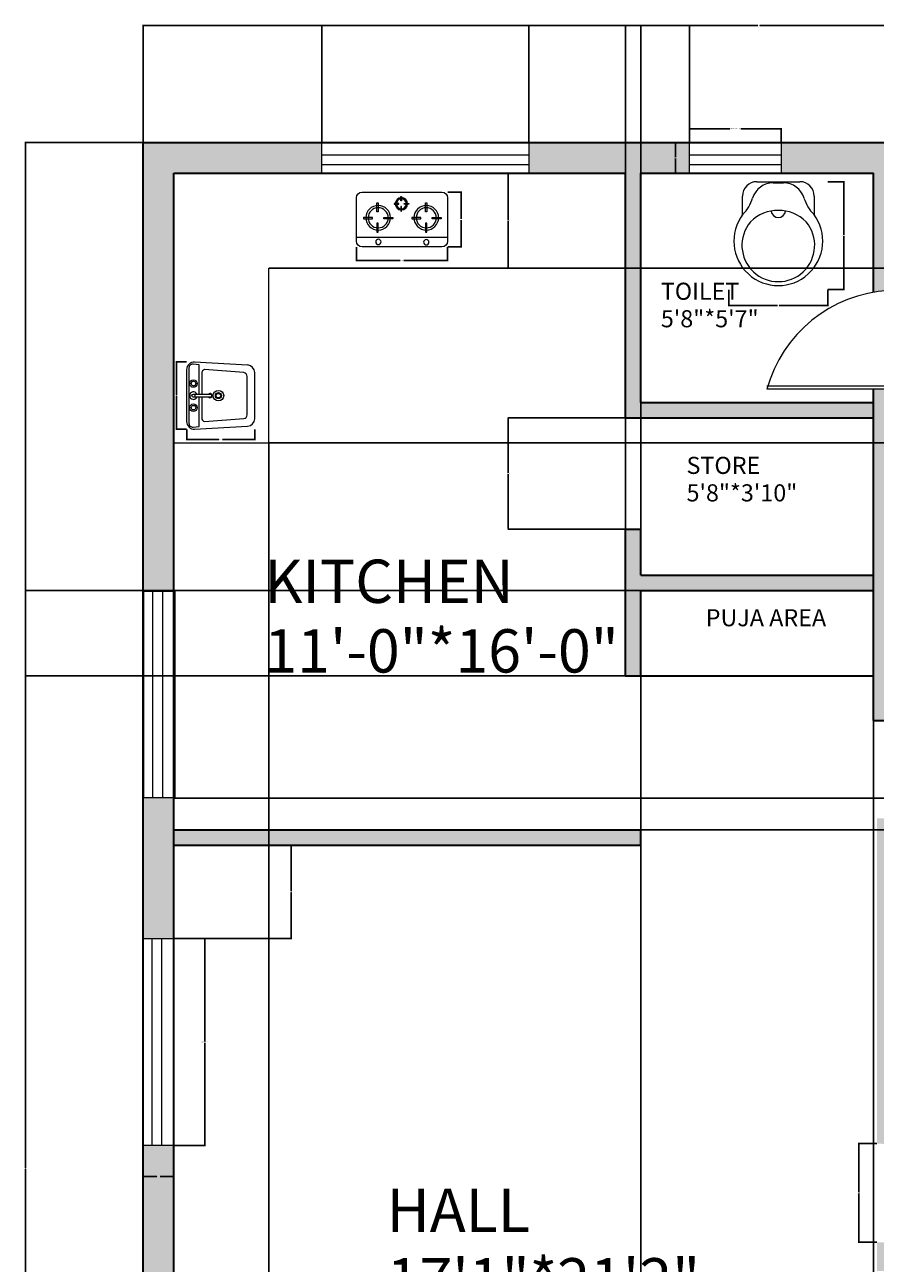
# Model space of a CAD drawing. Units: feet. Extents: x 2516 to 2945, y 1283 to 1993.
# Tile 2 of 3: x 2516 to 2764, y 1631 to 1993. Entities that reach past the tile are written whole.
import ezdxf

# ---------------------------------------------------------------- set-up
doc = ezdxf.new("R2010")
doc.units = ezdxf.units.FT
doc.layers.get('0').update_dxf_attribs({"lineweight": 18})
for name, color, linetype, lineweight in [('A-ANNO-DIMS', 2, 'Continuous', 18), ('A-AREA-IDEN', 7, 'Continuous', 18), ('A-EQPM', 8, 'Continuous', 18), ('A-FLOR-CASE', 8, 'Continuous', 18), ('A-FLOR-FIXT', 8, 'Continuous', 18), ('A-WALL', 7, 'Continuous', 35), ('A-WALL-PATT', 143, 'Continuous', 13), ('doors', 163, 'Continuous', 18), ('windows', 10, 'Continuous', 18)]:
    doc.layers.add(name, color=color, linetype=linetype, lineweight=lineweight)
doc.styles.get("Standard").update_dxf_attribs({"font": 'arial.ttf'})
doc.dimstyles.get("Standard").update_dxf_attribs({"dimtxt": 0.18, "dimasz": 0.18, "dimexe": 0.18, "dimexo": 0.0625, "dimgap": 0.09, "dimtad": 0, "dimtih": 1, "dimtoh": 1, "dimdec": 4, "dimzin": 0, "dimdsep": 46, "dimtxsty": 'Standard', "dimcen": 0.09, "dimadec": 0, "dimazin": 0, "dimtfac": 1, "dimtdec": 4, "dimtofl": 0, "dimtmove": 0, "dimatfit": 3, "dimfxl": 1, "dimtolj": 1, "dimtzin": 0, "dimarcsym": 0})

# ---------------------------------------------------------------- blocks, each defined once
blk = doc.blocks.new('door')
at = {"layer": 'doors'}
for p, q in [((-0.98, 0), (-0.98, 35.67)), ((0, 35.67), (0, 0)), ((-0.98, 0), (27.91, 0))]:
    blk.add_line(p, q, dxfattribs=at)
blk.add_arc((-11.23, -2.17), 39.2, 3.167, 74.8469, dxfattribs=at)
blk = doc.blocks.new('A$C39AA428E')
for p, q in [((0.4054, 0.435), (0.0392, 0.435)), ((0.3942, 0.45), (0.0499, 0.45)), ((0, 0.3972), (0.0194, 0.0472)), ((0.0143, 0.408), (0.0177, 0.3665)), ((0.0177, 0.3665), (0.2121, 0.3665)), ((0.05, 0.3311), (0.0702, 0.0729)), ((0.2121, 0.35), (0.0742, 0.35)), ((0.2121, 0.285), (0.2121, 0.405)), ((0.2321, 0.405), (0.2321, 0.285)), ((0.2321, 0.3665), (0.4265, 0.3665)), ((0.3699, 0.35), (0.2321, 0.35)), ((0.374, 0.0729), (0.3941, 0.3311)), ((0.4247, 0.0472), (0.4441, 0.3972)), ((0.4265, 0.3665), (0.4303, 0.4077)), ((0.2321, 0.285), (0.2121, 0.285)), ((0.0694, 0), (0.3748, 0)), ((0.0951, 0.05), (0.3491, 0.05))]:
    blk.add_line(p, q)
for centre, radius in [((0.1421, 0.405), 0.025), ((0.1421, 0.405), 0.015), ((0.2221, 0.405), 0.01), ((0.3021, 0.405), 0.025), ((0.3021, 0.405), 0.015), ((0.2221, 0.24), 0.035), ((0.2221, 0.24), 0.02), ((0.2221, 0.24), 0.015)]:
    blk.add_circle(centre, radius)
for centre, radius, start, end in [((0.0499, 0.4), 0.05, 90, 183.17983), ((0.0392, 0.41), 0.025, 90, 184.67219), ((0.2221, 0.405), 0.025, 293.57818, 246.42182), ((0.3942, 0.4), 0.05, 356.82017, 90), ((0.4054, 0.41), 0.025, 354.70992, 90), ((0.0742, 0.325), 0.025, 90, 165.81434), ((0.3699, 0.325), 0.025, 14.18566, 90), ((0.2221, 0.295), 0.0142, 134.62622, 45.19255), ((0.0694, 0.05), 0.05, 183.17983, 270), ((0.0951, 0.075), 0.025, 184.76364, 270), ((0.3491, 0.075), 0.025, 270, 355.23636), ((0.3748, 0.05), 0.05, 270, 356.82017)]:
    blk.add_arc(centre, radius, start, end)
blk = doc.blocks.new('A$C6EF51710')
at = {"linetype": 'ByBlock'}
for p, q in [((0.0508, 0.2843), (0.1169, 0.2843)), ((0, 0.0811), (0, 0.2335)), ((0.0041, 0.1392), (0.0041, 0.1755)), ((0.1169, 0.0303), (0.0508, 0.0303))]:
    blk.add_line(p, q, dxfattribs=at)
for centre, radius, start, end in [((0.2107, 0.1573), 0.1576, 232.8984, 127.1016), ((0.0508, 0.2335), 0.0508, 90, 180), ((0.0168, 0.3818), 0.1397, 287.1046, 315), ((0.2254, 0.1573), 0.1289, 230.0084, 129.9916), ((0.0803, 0.1755), 0.0762, 107.1046, 180), ((0.2413, 0.1573), 0.1397, 135, 225), ((0.1016, 0.1573), 0.0254, 275.2159, 84.7841), ((0.0803, 0.1392), 0.0762, 180, 252.8954), ((0.0508, 0.0811), 0.0508, 180, 270), ((0.0168, -0.0672), 0.1397, 45, 72.8954)]:
    blk.add_arc(centre, radius, start, end, dxfattribs=at)
blk = doc.blocks.new('A$C03A44EBA')
at = {"rotation": 270}
blk.add_blockref('A$C6EF51710', (0.0003, 0.3683), dxfattribs=at)
blk = doc.blocks.new('A$C2A3C6842')
for p, q in [((45, 432), (675, 432)), ((351.6, 363.3), (351.6, 398.9)), ((351.6, 398.9), (357.3, 398.9)), ((357.3, 398.9), (357.3, 363.3)), ((0, 45), (0, 387)), ((161.8, 346.9), (173.2, 346.9)), ((161.8, 275.6), (161.8, 346.9)), ((173.2, 346.9), (173.2, 275.6)), ((298.4, 341.9), (298.4, 336.2)), ((334, 341.9), (298.4, 341.9)), ((298.4, 336.2), (334, 336.2)), ((334, 336.2), (334, 341.9)), ((357.3, 363.3), (351.6, 363.3)), ((357.3, 318.8), (351.6, 318.8)), ((351.6, 318.8), (351.6, 283.1)), ((357.3, 283.1), (357.3, 318.8)), ((378.5, 336.2), (378.5, 341.9)), ((378.5, 341.9), (414.2, 341.9)), ((414.2, 336.2), (378.5, 336.2)), ((414.2, 341.9), (414.2, 336.2)), ((544.7, 346.9), (556.1, 346.9)), ((544.7, 275.6), (544.7, 346.9)), ((556.1, 346.9), (556.1, 275.6)), ((720, 387), (720, 45)), ((55.3, 232.9), (55.3, 221.5)), ((126.6, 232.9), (55.3, 232.9)), ((55.3, 221.5), (126.6, 221.5)), ((126.6, 221.5), (126.6, 232.9)), ((173.2, 275.6), (161.8, 275.6)), ((215.6, 221.5), (215.6, 232.9)), ((215.6, 232.9), (286.9, 232.9)), ((286.9, 221.5), (215.6, 221.5)), ((286.9, 232.9), (286.9, 221.5)), ((351.6, 283.1), (357.3, 283.1)), ((438.2, 232.9), (438.2, 221.5)), ((509.5, 232.9), (438.2, 232.9)), ((438.2, 221.5), (509.5, 221.5)), ((509.5, 221.5), (509.5, 232.9)), ((556.1, 275.6), (544.7, 275.6)), ((598.5, 232.9), (669.8, 232.9)), ((598.5, 221.5), (598.5, 232.9)), ((669.8, 221.5), (598.5, 221.5)), ((669.8, 232.9), (669.8, 221.5)), ((173.2, 186.6), (161.8, 186.6)), ((161.8, 186.6), (161.8, 115.3)), ((161.8, 115.3), (173.2, 115.3)), ((173.2, 115.3), (173.2, 186.6)), ((556.1, 186.6), (544.7, 186.6)), ((544.7, 186.6), (544.7, 115.3)), ((544.7, 115.3), (556.1, 115.3)), ((556.1, 115.3), (556.1, 186.6)), ((1.2, 76.7), (719.9, 76.7)), ((675, 0), (45, 0))]:
    blk.add_line(p, q)
at = {"extrusion": (0, -1e-16, -1)}
for centre, major_axis, start_param, end_param in [((45, 387), (31.8, 31.8), 3.926991, 5.497787), ((172.2, 229.8), (-97.3, 0.1), -0.001099, 6.282086), ((551.8, 229.8), (-97.3, 0.1), -0.001099, 6.282086), ((173.7, 39), (-14.8, 14.8), 5.497787, 11.780972)]:
    blk.add_ellipse(centre, major_axis=major_axis, ratio=1, start_param=start_param, end_param=end_param, dxfattribs=at)
at = {"extrusion": (0, 1e-16, -1)}
blk.add_ellipse((675, 387), major_axis=(-31.8, 31.8), ratio=1, start_param=0.785398, end_param=2.356194, dxfattribs=at)
at = {"extrusion": (-1e-16, -4e-16, -1)}
for centre in [(172.2, 229.8), (551.8, 229.8)]:
    blk.add_ellipse(centre, major_axis=(-79.3, 0), ratio=1, start_param=-0.0002116186602152, end_param=6.282973688519371, dxfattribs=at)
at = {"extrusion": (-1e-16, -1e-16, -1)}
blk.add_ellipse((355.1, 340.4), major_axis=(48.7, 0.1), ratio=1, start_param=3.144125, end_param=9.42731, dxfattribs=at)
at = {"extrusion": (-1e-16, 0, -1)}
for centre, major_axis, start_param, end_param in [((355.1, 340.4), (-39.7, 0), -0.000334, 6.282851), ((45, 45), (-31.8, 31.8), 3.926991, 5.497787)]:
    blk.add_ellipse(centre, major_axis=major_axis, ratio=1, start_param=start_param, end_param=end_param, dxfattribs=at)
at = {"extrusion": (2e-16, -2e-16, -1)}
blk.add_ellipse((551.4, 36.4), major_axis=(14.8, 14.8), ratio=1, start_param=3.926991, end_param=10.210176, dxfattribs=at)
at = {"extrusion": (-2e-16, 1e-16, -1)}
blk.add_ellipse((675, 45), major_axis=(31.8, 31.8), ratio=1, start_param=0.785398, end_param=2.356194, dxfattribs=at)
at = {"text_generation_flag": 4, "flags": 9}
for tag in ['XSIZE', 'YSIZE']:
    blk.add_attdef(tag, (361.3, 264.9), '', height=0.45, rotation=180, dxfattribs=at)
blk = doc.blocks.new('WIN-STANDARD')
for p, q in [((2.52, 60.52), (2.52, 0)), ((5.4, 60.52), (5.4, 0))]:
    blk.add_line(p, q)
blk.add_lwpolyline([(0, 60.52), (9, 60.52), (9, 0), (0, 0)], close=True)
blk = doc.blocks.new('WIN-TOILET')
for p, q in [((0, 5.4), (26.87, 5.4)), ((0, 2.52), (26.87, 2.52))]:
    blk.add_line(p, q)
blk.add_lwpolyline([(0, 9), (26.87, 9), (26.87, 0), (0, 0)], close=True)
blk = doc.blocks.new('*D9')
at = {"layer": 'A-ANNO-DIMS', "color": 0, "lineweight": -2, "transparency": 16777216}
for p, q in [((2559.48, 1726.05), (2568.67, 1726.05)), ((2568.49, 1725.87), (2568.49, 1695.97)), ((2568.49, 1665.71), (2568.49, 1695.6)), ((2559.48, 1665.53), (2568.67, 1665.53))]:
    blk.add_line(p, q, dxfattribs=at)
at = {"layer": 'A-ANNO-DIMS', "color": 0, "transparency": 16777216}
for points in [[(2568.46, 1725.87), (2568.52, 1725.87), (2568.49, 1726.05)], [(2568.46, 1665.71), (2568.52, 1665.71), (2568.49, 1665.53)]]:
    blk.add_solid(points, dxfattribs=at)
at = {"layer": 'Defpoints', "color": 0, "transparency": 16777216}
for p in [(2559.42, 1726.05), (2568.49, 1726.05), (2559.42, 1665.53)]:
    blk.add_point(p, dxfattribs=at)
at = {"layer": 'A-ANNO-DIMS', "color": 0, "transparency": 16777216, "insert": (2568.49, 1695.79), "char_height": 0.18, "attachment_point": 5}
blk.add_mtext('\\A1;WINDOW 61 TYP.', dxfattribs=at)
blk = doc.blocks.new('*D10')
at = {"layer": 'A-ANNO-DIMS', "color": 0, "lineweight": -2, "transparency": 16777216}
for p, q in [((2550.42, 1665.47), (2550.42, 1656.27)), ((2559.42, 1665.47), (2559.42, 1656.27)), ((2550.6, 1656.45), (2554.46, 1656.45)), ((2559.24, 1656.45), (2555.38, 1656.45))]:
    blk.add_line(p, q, dxfattribs=at)
at = {"layer": 'A-ANNO-DIMS', "color": 0, "transparency": 16777216}
for points in [[(2550.6, 1656.48), (2550.6, 1656.42), (2550.42, 1656.45)], [(2559.24, 1656.48), (2559.24, 1656.42), (2559.42, 1656.45)]]:
    blk.add_solid(points, dxfattribs=at)
at = {"layer": 'Defpoints', "color": 0, "transparency": 16777216}
for p in [(2550.42, 1665.53), (2559.42, 1665.53), (2559.42, 1656.45)]:
    blk.add_point(p, dxfattribs=at)
at = {"layer": 'A-ANNO-DIMS', "color": 0, "transparency": 16777216, "insert": (2554.92, 1656.45), "char_height": 0.18, "attachment_point": 5}
blk.add_mtext('\\A1;9 TYP.', dxfattribs=at)
blk = doc.blocks.new('*D11')
at = {"layer": 'A-ANNO-DIMS', "color": 0, "lineweight": -2, "transparency": 16777216}
for p, q in [((2710.09, 1958.92), (2710.09, 1963.07)), ((2736.96, 1958.92), (2736.96, 1963.07)), ((2710.27, 1962.89), (2721.94, 1962.89)), ((2736.78, 1962.89), (2725.12, 1962.89))]:
    blk.add_line(p, q, dxfattribs=at)
at = {"layer": 'A-ANNO-DIMS', "color": 0, "transparency": 16777216}
for points in [[(2710.27, 1962.92), (2710.27, 1962.86), (2710.09, 1962.89)], [(2736.78, 1962.92), (2736.78, 1962.86), (2736.96, 1962.89)]]:
    blk.add_solid(points, dxfattribs=at)
at = {"layer": 'Defpoints', "color": 0, "transparency": 16777216}
for p in [(2736.96, 1962.89), (2710.09, 1958.86), (2736.96, 1958.86)]:
    blk.add_point(p, dxfattribs=at)
at = {"layer": 'A-ANNO-DIMS', "color": 0, "transparency": 16777216, "insert": (2723.53, 1962.89), "char_height": 0.18, "attachment_point": 5}
blk.add_mtext('\\A1;TOILET WINDOW 27 TYP.', dxfattribs=at)
blk = doc.blocks.new('*D12')
at = {"layer": 'A-ANNO-DIMS', "color": 0, "lineweight": -2, "transparency": 16777216}
for p, q in [((2710.03, 1958.86), (2705.88, 1958.86)), ((2706.06, 1958.68), (2706.06, 1954.54)), ((2706.06, 1950.04), (2706.06, 1954.18)), ((2710.03, 1949.86), (2705.88, 1949.86))]:
    blk.add_line(p, q, dxfattribs=at)
at = {"layer": 'A-ANNO-DIMS', "color": 0, "transparency": 16777216}
for points in [[(2706.03, 1958.68), (2706.09, 1958.68), (2706.06, 1958.86)], [(2706.03, 1950.04), (2706.09, 1950.04), (2706.06, 1949.86)]]:
    blk.add_solid(points, dxfattribs=at)
at = {"layer": 'Defpoints', "color": 0, "transparency": 16777216}
for p in [(2706.06, 1958.86), (2710.09, 1958.86), (2710.09, 1949.86)]:
    blk.add_point(p, dxfattribs=at)
at = {"layer": 'A-ANNO-DIMS', "color": 0, "transparency": 16777216, "insert": (2706.06, 1954.36), "char_height": 0.18, "attachment_point": 5}
blk.add_mtext('\\A1;9 TYP.', dxfattribs=at)
blk = doc.blocks.new('*D14')
at = {"layer": 'A-ANNO-DIMS', "color": 0, "lineweight": -2, "transparency": 16777216}
for p, q in [((2764.9, 1666.13), (2759.43, 1666.13)), ((2759.61, 1665.95), (2759.61, 1651.86)), ((2759.61, 1637.42), (2759.61, 1651.5)), ((2764.9, 1637.24), (2759.43, 1637.24))]:
    blk.add_line(p, q, dxfattribs=at)
at = {"layer": 'A-ANNO-DIMS', "color": 0, "transparency": 16777216}
for points in [[(2759.58, 1665.95), (2759.64, 1665.95), (2759.61, 1666.13)], [(2759.58, 1637.42), (2759.64, 1637.42), (2759.61, 1637.24)]]:
    blk.add_solid(points, dxfattribs=at)
at = {"layer": 'Defpoints', "color": 0, "transparency": 16777216}
for p in [(2759.61, 1666.13), (2764.96, 1666.13), (2764.96, 1637.24)]:
    blk.add_point(p, dxfattribs=at)
at = {"layer": 'A-ANNO-DIMS', "color": 0, "transparency": 16777216, "insert": (2759.61, 1651.68), "char_height": 0.18, "attachment_point": 5}
blk.add_mtext('\\A1;29 TYP.', dxfattribs=at)
blk = doc.blocks.new('*D19')
at = {"layer": 'A-ANNO-DIMS', "color": 0, "lineweight": -2, "transparency": 16777216}
for p, q in [((2750.58, 1947.39), (2755.42, 1947.39)), ((2755.24, 1947.21), (2755.24, 1931.82)), ((2755.24, 1916.06), (2755.24, 1931.45)), ((2750.58, 1915.88), (2755.42, 1915.88))]:
    blk.add_line(p, q, dxfattribs=at)
at = {"layer": 'A-ANNO-DIMS', "color": 0, "transparency": 16777216}
for points in [[(2755.21, 1947.21), (2755.27, 1947.21), (2755.24, 1947.39)], [(2755.21, 1916.06), (2755.27, 1916.06), (2755.24, 1915.88)]]:
    blk.add_solid(points, dxfattribs=at)
at = {"layer": 'Defpoints', "color": 0, "transparency": 16777216}
for p in [(2750.52, 1947.39), (2755.24, 1947.39), (2750.52, 1915.88)]:
    blk.add_point(p, dxfattribs=at)
at = {"layer": 'A-ANNO-DIMS', "color": 0, "transparency": 16777216, "insert": (2755.24, 1931.64), "char_height": 0.18, "attachment_point": 5}
blk.add_mtext('\\A1;WC 32', dxfattribs=at)
blk = doc.blocks.new('*D20')
at = {"layer": 'A-ANNO-DIMS', "color": 0, "lineweight": -2, "transparency": 16777216}
for p, q in [((2721.67, 1915.82), (2721.67, 1910.97)), ((2750.52, 1915.82), (2750.52, 1910.97)), ((2721.85, 1911.15), (2735.87, 1911.15)), ((2750.34, 1911.15), (2736.31, 1911.15))]:
    blk.add_line(p, q, dxfattribs=at)
at = {"layer": 'A-ANNO-DIMS', "color": 0, "transparency": 16777216}
for points in [[(2721.85, 1911.18), (2721.85, 1911.12), (2721.67, 1911.15)], [(2750.34, 1911.18), (2750.34, 1911.12), (2750.52, 1911.15)]]:
    blk.add_solid(points, dxfattribs=at)
at = {"layer": 'Defpoints', "color": 0, "transparency": 16777216}
for p in [(2721.67, 1915.88), (2750.52, 1915.88), (2750.52, 1911.15)]:
    blk.add_point(p, dxfattribs=at)
at = {"layer": 'A-ANNO-DIMS', "color": 0, "transparency": 16777216, "insert": (2736.09, 1911.15), "char_height": 0.18, "attachment_point": 5}
blk.add_mtext('\\A1;29', dxfattribs=at)
blk = doc.blocks.new('*D23')
at = {"layer": 'A-ANNO-DIMS', "color": 0, "lineweight": -2, "transparency": 16777216}
for p, q in [((2563.15, 1874.92), (2563.15, 1871.82)), ((2583.04, 1874.92), (2583.04, 1871.82)), ((2563.33, 1872), (2572.55, 1872)), ((2582.86, 1872), (2573.64, 1872))]:
    blk.add_line(p, q, dxfattribs=at)
at = {"layer": 'A-ANNO-DIMS', "color": 0, "transparency": 16777216}
for points in [[(2563.33, 1872.03), (2563.33, 1871.97), (2563.15, 1872)], [(2582.86, 1872.03), (2582.86, 1871.97), (2583.04, 1872)]]:
    blk.add_solid(points, dxfattribs=at)
at = {"layer": 'Defpoints', "color": 0, "transparency": 16777216}
for p in [(2563.15, 1874.98), (2583.04, 1874.98), (2563.15, 1872)]:
    blk.add_point(p, dxfattribs=at)
at = {"layer": 'A-ANNO-DIMS', "color": 0, "transparency": 16777216, "insert": (2573.09, 1872), "char_height": 0.18, "attachment_point": 5}
blk.add_mtext('\\A1;SINK 20', dxfattribs=at)
blk = doc.blocks.new('*D24')
at = {"layer": 'A-ANNO-DIMS', "color": 0, "lineweight": -2, "transparency": 16777216}
for p, q in [((2563.08, 1894.68), (2559.98, 1894.68)), ((2560.16, 1894.5), (2560.16, 1885.01)), ((2560.16, 1875.16), (2560.16, 1884.65)), ((2563.08, 1874.98), (2559.98, 1874.98))]:
    blk.add_line(p, q, dxfattribs=at)
at = {"layer": 'A-ANNO-DIMS', "color": 0, "transparency": 16777216}
for points in [[(2560.13, 1894.5), (2560.19, 1894.5), (2560.16, 1894.68)], [(2560.13, 1875.16), (2560.19, 1875.16), (2560.16, 1874.98)]]:
    blk.add_solid(points, dxfattribs=at)
at = {"layer": 'Defpoints', "color": 0, "transparency": 16777216}
for p in [(2560.16, 1894.68), (2563.15, 1894.68), (2563.15, 1874.98)]:
    blk.add_point(p, dxfattribs=at)
at = {"layer": 'A-ANNO-DIMS', "color": 0, "transparency": 16777216, "insert": (2560.16, 1884.83), "char_height": 0.18, "attachment_point": 5}
blk.add_mtext('\\A1;20', dxfattribs=at)
blk = doc.blocks.new('*D25')
at = {"layer": 'A-ANNO-DIMS', "color": 0, "lineweight": -2, "transparency": 16777216}
for p, q in [((2612.76, 1928.28), (2612.76, 1924.16)), ((2639.41, 1928.28), (2639.41, 1924.16)), ((2612.94, 1924.34), (2625.56, 1924.34)), ((2639.23, 1924.34), (2626.61, 1924.34))]:
    blk.add_line(p, q, dxfattribs=at)
at = {"layer": 'A-ANNO-DIMS', "color": 0, "transparency": 16777216}
for points in [[(2612.94, 1924.37), (2612.94, 1924.31), (2612.76, 1924.34)], [(2639.23, 1924.37), (2639.23, 1924.31), (2639.41, 1924.34)]]:
    blk.add_solid(points, dxfattribs=at)
at = {"layer": 'Defpoints', "color": 0, "transparency": 16777216}
for p in [(2612.76, 1928.34), (2639.41, 1928.34), (2639.41, 1924.34)]:
    blk.add_point(p, dxfattribs=at)
at = {"layer": 'A-ANNO-DIMS', "color": 0, "transparency": 16777216, "insert": (2626.09, 1924.34), "char_height": 0.18, "attachment_point": 5}
blk.add_mtext('\\A1;HOB 27', dxfattribs=at)
blk = doc.blocks.new('*D26')
at = {"layer": 'A-ANNO-DIMS', "color": 0, "lineweight": -2, "transparency": 16777216}
for p, q in [((2639.48, 1944.33), (2643.59, 1944.33)), ((2643.41, 1944.15), (2643.41, 1936.52)), ((2643.41, 1928.52), (2643.41, 1936.15)), ((2639.48, 1928.34), (2643.59, 1928.34))]:
    blk.add_line(p, q, dxfattribs=at)
at = {"layer": 'A-ANNO-DIMS', "color": 0, "transparency": 16777216}
for points in [[(2643.38, 1944.15), (2643.44, 1944.15), (2643.41, 1944.33)], [(2643.38, 1928.52), (2643.44, 1928.52), (2643.41, 1928.34)]]:
    blk.add_solid(points, dxfattribs=at)
at = {"layer": 'Defpoints', "color": 0, "transparency": 16777216}
for p in [(2639.41, 1944.33), (2643.41, 1944.33), (2639.41, 1928.34)]:
    blk.add_point(p, dxfattribs=at)
at = {"layer": 'A-ANNO-DIMS', "color": 0, "transparency": 16777216, "insert": (2643.41, 1936.34), "char_height": 0.18, "attachment_point": 5}
blk.add_mtext('\\A1;16', dxfattribs=at)
blk = doc.blocks.new('*D27')
at = {"layer": 'A-ANNO-DIMS', "color": 0, "lineweight": -2, "transparency": 16777216}
for p, q in [((2550.42, 1958.92), (2550.42, 1993.29)), ((2550.6, 1993.11), (2730.13, 1993.11)), ((2910.24, 1993.11), (2730.71, 1993.11)), ((2910.42, 1958.92), (2910.42, 1993.29))]:
    blk.add_line(p, q, dxfattribs=at)
at = {"layer": 'A-ANNO-DIMS', "color": 0, "transparency": 16777216}
for points in [[(2550.6, 1993.14), (2550.6, 1993.08), (2550.42, 1993.11)], [(2910.24, 1993.14), (2910.24, 1993.08), (2910.42, 1993.11)]]:
    blk.add_solid(points, dxfattribs=at)
at = {"layer": 'Defpoints', "color": 0, "transparency": 16777216}
for p in [(2910.42, 1993.11), (2550.42, 1958.86), (2910.42, 1958.86)]:
    blk.add_point(p, dxfattribs=at)
at = {"layer": 'A-ANNO-DIMS', "color": 0, "transparency": 16777216, "insert": (2730.42, 1993.11), "char_height": 0.18, "attachment_point": 5}
blk.add_mtext('\\A1;360', dxfattribs=at)
blk = doc.blocks.new('*D28')
at = {"layer": 'A-ANNO-DIMS', "color": 0, "lineweight": -2, "transparency": 16777216}
for p, q in [((2550.35, 1958.86), (2515.85, 1958.86)), ((2516.03, 1958.68), (2516.03, 1659.04)), ((2516.03, 1359.04), (2516.03, 1658.68)), ((2550.35, 1358.86), (2515.85, 1358.86))]:
    blk.add_line(p, q, dxfattribs=at)
at = {"layer": 'A-ANNO-DIMS', "color": 0, "transparency": 16777216}
for points in [[(2516, 1958.68), (2516.06, 1958.68), (2516.03, 1958.86)], [(2516, 1359.04), (2516.06, 1359.04), (2516.03, 1358.86)]]:
    blk.add_solid(points, dxfattribs=at)
at = {"layer": 'Defpoints', "color": 0, "transparency": 16777216}
for p in [(2516.03, 1958.86), (2550.42, 1958.86), (2550.42, 1358.86)]:
    blk.add_point(p, dxfattribs=at)
at = {"layer": 'A-ANNO-DIMS', "color": 0, "transparency": 16777216, "insert": (2516.03, 1658.86), "char_height": 0.18, "attachment_point": 5}
blk.add_mtext('\\A1;600', dxfattribs=at)
blk = doc.blocks.new('*D29')
at = {"layer": 'A-ANNO-DIMS', "color": 0, "lineweight": -2, "transparency": 16777216}
for p, q in [((2550.42, 1958.92), (2550.42, 1993.29)), ((2550.6, 1993.11), (2576.15, 1993.11)), ((2602.49, 1993.11), (2576.94, 1993.11)), ((2602.67, 1958.92), (2602.67, 1993.29))]:
    blk.add_line(p, q, dxfattribs=at)
at = {"layer": 'A-ANNO-DIMS', "color": 0, "transparency": 16777216}
for points in [[(2550.6, 1993.14), (2550.6, 1993.08), (2550.42, 1993.11)], [(2602.49, 1993.14), (2602.49, 1993.08), (2602.67, 1993.11)]]:
    blk.add_solid(points, dxfattribs=at)
at = {"layer": 'Defpoints', "color": 0, "transparency": 16777216}
for p in [(2602.67, 1993.11), (2550.42, 1958.86), (2602.67, 1958.86)]:
    blk.add_point(p, dxfattribs=at)
at = {"layer": 'A-ANNO-DIMS', "color": 0, "transparency": 16777216, "insert": (2576.54, 1993.11), "char_height": 0.18, "attachment_point": 5}
blk.add_mtext('\\A1;52.25', dxfattribs=at)
blk = doc.blocks.new('*D30')
at = {"layer": 'A-ANNO-DIMS', "color": 0, "lineweight": -2, "transparency": 16777216}
for p, q in [((2663.19, 1958.92), (2663.19, 1993.29)), ((2663.37, 1993.11), (2686.31, 1993.11)), ((2709.91, 1993.11), (2686.97, 1993.11)), ((2710.09, 1958.92), (2710.09, 1993.29))]:
    blk.add_line(p, q, dxfattribs=at)
at = {"layer": 'A-ANNO-DIMS', "color": 0, "transparency": 16777216}
for points in [[(2663.37, 1993.14), (2663.37, 1993.08), (2663.19, 1993.11)], [(2709.91, 1993.14), (2709.91, 1993.08), (2710.09, 1993.11)]]:
    blk.add_solid(points, dxfattribs=at)
at = {"layer": 'Defpoints', "color": 0, "transparency": 16777216}
for p in [(2710.09, 1993.11), (2663.19, 1958.86), (2710.09, 1958.86)]:
    blk.add_point(p, dxfattribs=at)
at = {"layer": 'A-ANNO-DIMS', "color": 0, "transparency": 16777216, "insert": (2686.64, 1993.11), "char_height": 0.18, "attachment_point": 5}
blk.add_mtext('\\A1;46.9', dxfattribs=at)
blk = doc.blocks.new('*D33')
at = {"layer": 'A-ANNO-DIMS', "color": 0, "lineweight": -2, "transparency": 16777216}
for p, q in [((2559.48, 1753.36), (2593.85, 1753.36)), ((2593.67, 1753.18), (2593.67, 1739.88)), ((2593.67, 1726.23), (2593.67, 1739.52)), ((2559.48, 1726.05), (2593.85, 1726.05))]:
    blk.add_line(p, q, dxfattribs=at)
at = {"layer": 'A-ANNO-DIMS', "color": 0, "transparency": 16777216}
for points in [[(2593.64, 1753.18), (2593.7, 1753.18), (2593.67, 1753.36)], [(2593.64, 1726.23), (2593.7, 1726.23), (2593.67, 1726.05)]]:
    blk.add_solid(points, dxfattribs=at)
at = {"layer": 'Defpoints', "color": 0, "transparency": 16777216}
for p in [(2559.42, 1753.36), (2559.42, 1726.05), (2593.67, 1726.05)]:
    blk.add_point(p, dxfattribs=at)
at = {"layer": 'A-ANNO-DIMS', "color": 0, "transparency": 16777216, "insert": (2593.67, 1739.7), "char_height": 0.18, "attachment_point": 5}
blk.add_mtext('\\A1;27.31', dxfattribs=at)
blk = doc.blocks.new('*D34')
at = {"layer": 'A-ANNO-DIMS', "color": 0, "lineweight": -2, "transparency": 16777216}
for p, q in [((2559.71, 1767.16), (2945.03, 1767.16)), ((2944.85, 1766.98), (2944.85, 1762.69)), ((2944.85, 1758.04), (2944.85, 1762.33)), ((2559.48, 1757.86), (2945.03, 1757.86))]:
    blk.add_line(p, q, dxfattribs=at)
at = {"layer": 'A-ANNO-DIMS', "color": 0, "transparency": 16777216}
for points in [[(2944.82, 1766.98), (2944.88, 1766.98), (2944.85, 1767.16)], [(2944.82, 1758.04), (2944.88, 1758.04), (2944.85, 1757.86)]]:
    blk.add_solid(points, dxfattribs=at)
at = {"layer": 'Defpoints', "color": 0, "transparency": 16777216}
for p in [(2559.64, 1767.16), (2944.85, 1767.16), (2559.42, 1757.86)]:
    blk.add_point(p, dxfattribs=at)
at = {"layer": 'A-ANNO-DIMS', "color": 0, "transparency": 16777216, "insert": (2944.85, 1762.51), "char_height": 0.18, "attachment_point": 5}
blk.add_mtext('\\A1;9.306', dxfattribs=at)
blk = doc.blocks.new('*D43')
at = {"layer": 'A-ANNO-DIMS', "color": 0, "lineweight": -2, "transparency": 16777216}
for p, q in [((2695.92, 1802.8), (2695.92, 1324.43)), ((2763.92, 1802.8), (2763.92, 1324.43)), ((2696.1, 1324.61), (2729.7, 1324.61)), ((2763.74, 1324.61), (2730.14, 1324.61))]:
    blk.add_line(p, q, dxfattribs=at)
at = {"layer": 'A-ANNO-DIMS', "color": 0, "transparency": 16777216}
for points in [[(2696.1, 1324.64), (2696.1, 1324.58), (2695.92, 1324.61)], [(2763.74, 1324.64), (2763.74, 1324.58), (2763.92, 1324.61)]]:
    blk.add_solid(points, dxfattribs=at)
at = {"layer": 'Defpoints', "color": 0, "transparency": 16777216}
for p in [(2695.92, 1802.86), (2763.92, 1802.86), (2763.92, 1324.61)]:
    blk.add_point(p, dxfattribs=at)
at = {"layer": 'A-ANNO-DIMS', "color": 0, "transparency": 16777216, "insert": (2729.92, 1324.61), "char_height": 0.18, "attachment_point": 5}
blk.add_mtext('\\A1;68', dxfattribs=at)
blk = doc.blocks.new('*D44')
at = {"layer": 'A-ANNO-DIMS', "color": 0, "lineweight": -2, "transparency": 16777216}
for p, q in [((2695.85, 1827.86), (2515.85, 1827.86)), ((2516.03, 1827.68), (2516.03, 1815.54)), ((2516.03, 1803.04), (2516.03, 1815.18)), ((2695.85, 1802.86), (2515.85, 1802.86))]:
    blk.add_line(p, q, dxfattribs=at)
at = {"layer": 'A-ANNO-DIMS', "color": 0, "transparency": 16777216}
for points in [[(2516, 1827.68), (2516.06, 1827.68), (2516.03, 1827.86)], [(2516, 1803.04), (2516.06, 1803.04), (2516.03, 1802.86)]]:
    blk.add_solid(points, dxfattribs=at)
at = {"layer": 'Defpoints', "color": 0, "transparency": 16777216}
for p in [(2516.03, 1827.86), (2695.92, 1827.86), (2695.92, 1802.86)]:
    blk.add_point(p, dxfattribs=at)
at = {"layer": 'A-ANNO-DIMS', "color": 0, "transparency": 16777216, "insert": (2516.03, 1815.36), "char_height": 0.18, "attachment_point": 5}
blk.add_mtext('\\A1;25', dxfattribs=at)
blk = doc.blocks.new('*D46')
at = {"layer": 'A-ANNO-DIMS', "color": 0, "lineweight": -2, "transparency": 16777216}
for p, q in [((2559.42, 1870.95), (2559.42, 1324.43)), ((2587.15, 1870.95), (2587.15, 1324.43)), ((2559.6, 1324.61), (2572.89, 1324.61)), ((2586.97, 1324.61), (2573.68, 1324.61))]:
    blk.add_line(p, q, dxfattribs=at)
at = {"layer": 'A-ANNO-DIMS', "color": 0, "transparency": 16777216}
for points in [[(2559.6, 1324.64), (2559.6, 1324.58), (2559.42, 1324.61)], [(2586.97, 1324.64), (2586.97, 1324.58), (2587.15, 1324.61)]]:
    blk.add_solid(points, dxfattribs=at)
at = {"layer": 'Defpoints', "color": 0, "transparency": 16777216}
for p in [(2559.42, 1871.01), (2587.15, 1871.01), (2587.15, 1324.61)]:
    blk.add_point(p, dxfattribs=at)
at = {"layer": 'A-ANNO-DIMS', "color": 0, "transparency": 16777216, "insert": (2573.29, 1324.61), "char_height": 0.18, "attachment_point": 5}
blk.add_mtext('\\A1;27.74', dxfattribs=at)
blk = doc.blocks.new('*D47')
at = {"layer": 'A-ANNO-DIMS', "color": 0, "lineweight": -2, "transparency": 16777216}
for p, q in [((2587.22, 1922.13), (2945.03, 1922.13)), ((2944.85, 1921.95), (2944.85, 1896.75)), ((2944.85, 1871.19), (2944.85, 1896.39)), ((2587.22, 1871.01), (2945.03, 1871.01))]:
    blk.add_line(p, q, dxfattribs=at)
at = {"layer": 'A-ANNO-DIMS', "color": 0, "transparency": 16777216}
for points in [[(2944.82, 1921.95), (2944.88, 1921.95), (2944.85, 1922.13)], [(2944.82, 1871.19), (2944.88, 1871.19), (2944.85, 1871.01)]]:
    blk.add_solid(points, dxfattribs=at)
at = {"layer": 'Defpoints', "color": 0, "transparency": 16777216}
for p in [(2587.15, 1922.13), (2587.15, 1871.01), (2944.85, 1871.01)]:
    blk.add_point(p, dxfattribs=at)
at = {"layer": 'A-ANNO-DIMS', "color": 0, "transparency": 16777216, "insert": (2944.85, 1896.57), "char_height": 0.18, "attachment_point": 5}
blk.add_mtext('\\A1;51.12', dxfattribs=at)
blk = doc.blocks.new('*D49')
at = {"layer": 'A-ANNO-DIMS', "color": 0, "lineweight": -2, "transparency": 16777216}
for p, q in [((2691.35, 1949.86), (2656.99, 1949.86)), ((2657.17, 1949.68), (2657.17, 1936.17)), ((2657.17, 1922.31), (2657.17, 1935.81)), ((2691.35, 1922.13), (2656.99, 1922.13))]:
    blk.add_line(p, q, dxfattribs=at)
at = {"layer": 'A-ANNO-DIMS', "color": 0, "transparency": 16777216}
for points in [[(2657.14, 1949.68), (2657.2, 1949.68), (2657.17, 1949.86)], [(2657.14, 1922.31), (2657.2, 1922.31), (2657.17, 1922.13)]]:
    blk.add_solid(points, dxfattribs=at)
at = {"layer": 'Defpoints', "color": 0, "transparency": 16777216}
for p in [(2657.17, 1949.86), (2691.42, 1949.86), (2691.42, 1922.13)]:
    blk.add_point(p, dxfattribs=at)
at = {"layer": 'A-ANNO-DIMS', "color": 0, "transparency": 16777216, "insert": (2657.17, 1935.99), "char_height": 0.18, "attachment_point": 5}
blk.add_mtext('\\A1;27.727', dxfattribs=at)
blk = doc.blocks.new('*D50')
at = {"layer": 'A-ANNO-DIMS', "color": 0, "lineweight": -2, "transparency": 16777216}
for p, q in [((2691.35, 1878.36), (2656.99, 1878.36)), ((2657.17, 1878.18), (2657.17, 1862.27)), ((2657.17, 1845.99), (2657.17, 1861.9)), ((2691.35, 1845.81), (2656.99, 1845.81))]:
    blk.add_line(p, q, dxfattribs=at)
at = {"layer": 'A-ANNO-DIMS', "color": 0, "transparency": 16777216}
for points in [[(2657.14, 1878.18), (2657.2, 1878.18), (2657.17, 1878.36)], [(2657.14, 1845.99), (2657.2, 1845.99), (2657.17, 1845.81)]]:
    blk.add_solid(points, dxfattribs=at)
at = {"layer": 'Defpoints', "color": 0, "transparency": 16777216}
for p in [(2657.17, 1878.36), (2691.42, 1878.36), (2691.42, 1845.81)]:
    blk.add_point(p, dxfattribs=at)
at = {"layer": 'A-ANNO-DIMS', "color": 0, "transparency": 16777216, "insert": (2657.17, 1862.09), "char_height": 0.18, "attachment_point": 5}
blk.add_mtext('\\A1;32.544', dxfattribs=at)
blk = doc.blocks.new('*D51')
at = {"layer": 'A-ANNO-DIMS', "color": 0, "lineweight": -2, "transparency": 16777216}
for p, q in [((2691.42, 1845.88), (2691.42, 1993.29)), ((2691.6, 1993.11), (2693.41, 1993.11)), ((2695.74, 1993.11), (2693.93, 1993.11)), ((2695.92, 1845.88), (2695.92, 1993.29))]:
    blk.add_line(p, q, dxfattribs=at)
at = {"layer": 'A-ANNO-DIMS', "color": 0, "transparency": 16777216}
for points in [[(2691.6, 1993.14), (2691.6, 1993.08), (2691.42, 1993.11)], [(2695.74, 1993.14), (2695.74, 1993.08), (2695.92, 1993.11)]]:
    blk.add_solid(points, dxfattribs=at)
at = {"layer": 'Defpoints', "color": 0, "transparency": 16777216}
for p in [(2695.92, 1993.11), (2691.42, 1845.81), (2695.92, 1845.81)]:
    blk.add_point(p, dxfattribs=at)
at = {"layer": 'A-ANNO-DIMS', "color": 0, "transparency": 16777216, "insert": (2693.67, 1993.11), "char_height": 0.18, "attachment_point": 5}
blk.add_mtext('\\A1;4.5', dxfattribs=at)

msp = doc.modelspace()

# ---------------------------------------------------------------- hatches: boundary and pattern name
at = {"layer": 'A-WALL-PATT'}
h = msp.add_hatch(color=256, dxfattribs=at)
h.dxf.hatch_style = 1
h.paths.add_polyline_path([(2763.9169, 1832.358), (2695.9169, 1832.358), (2695.9169, 1845.8137), (2691.4169, 1845.8137), (2691.4169, 1802.858), (2695.9169, 1802.858), (2695.9169, 1827.858), (2763.9169, 1827.858)])
h.paths.add_polyline_path([(2768.4169, 1886.6758), (2763.9169, 1886.6758), (2763.9169, 1789.8455), (2764.9169, 1789.8455), (2764.9169, 1790.0678, -0.01619533), (2767.4458, 1789.8455), (2768.4169, 1789.8455)])
h.paths.add_polyline_path([(2710.0911, 1958.858), (2663.1874, 1958.858), (2663.1874, 1949.858), (2691.4169, 1949.858), (2691.4169, 1878.358), (2763.9169, 1878.358), (2763.9169, 1882.858), (2695.9169, 1882.858), (2695.9169, 1949.858), (2710.0911, 1949.858)])
h.paths.add_polyline_path([(2910.4169, 1958.858), (2736.9631, 1958.858), (2736.9631, 1949.858), (2763.9169, 1949.858), (2763.9169, 1915.057, -0.02890868), (2768.4169, 1915.568), (2768.4169, 1949.858), (2901.4169, 1949.858), (2901.4169, 1859.2593), (2910.4169, 1859.2593)])
h.paths.add_polyline_path([(2910.4169, 1798.7389), (2901.4169, 1798.7389), (2901.4169, 1757.858), (2769.4169, 1757.858), (2769.4169, 1761.1755), (2764.9169, 1761.1755), (2764.9596, 1666.1291, -0.0286323), (2769.4169, 1665.6254), (2769.4169, 1753.358), (2901.4169, 1753.358), (2901.4169, 1723.6182), (2910.4169, 1723.6182)])
h.paths.add_polyline_path([(2910.4169, 1663.0978), (2901.4169, 1663.0978), (2901.4169, 1633.358), (2769.4169, 1633.358), (2769.4169, 1637.2369), (2764.9596, 1637.2369), (2764.9596, 1628.858), (2901.4169, 1628.858), (2901.4169, 1610.8331), (2910.4169, 1610.8331)])
h.paths.add_polyline_path([(2910.4169, 1572.5822), (2901.4169, 1572.5822), (2901.4169, 1552.858), (2812.9169, 1552.858), (2812.9169, 1548.358), (2817.4169, 1548.358), (2901.4169, 1548.358), (2901.4169, 1534.5783), (2910.4169, 1534.5783)])
h.paths.add_polyline_path([(2910.4169, 1507.7063), (2901.4169, 1507.7063), (2901.4169, 1500.358), (2817.4169, 1500.358), (2817.4169, 1518.131, -0.02890927), (2812.9169, 1517.6191), (2812.9169, 1500.358), (2803.3072, 1500.358, -0.02890868), (2802.7962, 1495.858), (2901.4169, 1495.858), (2901.4169, 1367.858), (2881.9751, 1367.858), (2881.9751, 1358.858), (2910.4169, 1358.858)])
h.paths.add_polyline_path([(2821.4547, 1367.858), (2769.4169, 1367.858), (2769.4169, 1495.858), (2774.415, 1495.858), (2774.415, 1500.358), (2760.4256, 1500.358), (2760.4256, 1495.858), (2764.9169, 1495.858), (2764.9169, 1367.858), (2764.9169, 1358.858), (2821.4547, 1358.858)])
h.paths.add_polyline_path([(2731.4104, 1499.858), (2559.4169, 1499.858), (2559.4169, 1495.358), (2731.4104, 1495.358)])
h.paths.add_polyline_path([(2559.4169, 1665.5276), (2550.4169, 1665.5276), (2550.4169, 1577.9069), (2559.4169, 1577.9069)])
h.paths.add_polyline_path([(2559.4169, 1767.1637), (2550.4169, 1767.1637), (2550.4169, 1726.0479), (2559.4169, 1726.0479)])
h.paths.add_polyline_path([(2695.9169, 1757.858), (2559.4169, 1757.858), (2559.4169, 1753.358), (2695.9169, 1753.358)])
h.paths.add_polyline_path([(2559.4169, 1949.858), (2602.667, 1949.858), (2602.667, 1958.858), (2550.4169, 1958.858), (2550.4169, 1827.6841), (2559.4169, 1827.6841)])

# ---------------------------------------------------------------- linework, layer by layer
at = {"layer": 'A-FLOR-CASE'}
for p, q in [((2587.155, 1871.0142), (2587.155, 1922.1312)), ((2587.155, 1922.1312), (2691.4169, 1922.1312)), ((2559.4169, 1871.0142), (2587.155, 1871.0142))]:
    msp.add_line(p, q, dxfattribs=at)
at = {"layer": 'A-WALL'}
for p, q in [((2550.4169, 1958.858), (2910.4169, 1958.858)), ((2550.4169, 1358.858), (2550.4169, 1958.858)), ((2559.4169, 1949.858), (2691.4169, 1949.858)), ((2559.4169, 1499.858), (2559.4169, 1949.858)), ((2691.4169, 1878.358), (2691.4169, 1949.858)), ((2695.9169, 1949.858), (2763.9169, 1949.858)), ((2695.9169, 1882.858), (2695.9169, 1949.858)), ((2763.9169, 1915.057), (2763.9169, 1949.858)), ((2763.9169, 1915.057), (2763.9169, 1949.858)), ((2763.9169, 1882.858), (2763.9169, 1886.6758)), ((2763.9169, 1789.8455), (2763.9169, 1886.6758)), ((2695.9169, 1882.858), (2763.9169, 1882.858)), ((2691.4169, 1878.358), (2763.9169, 1878.358)), ((2763.9169, 1799.9415), (2763.9169, 1878.358)), ((2691.4169, 1802.858), (2691.4169, 1845.8137)), ((2691.4169, 1845.8137), (2695.9169, 1845.8137)), ((2695.9169, 1832.358), (2695.9169, 1845.8137)), ((2695.9169, 1832.358), (2763.9169, 1832.358)), ((2695.9169, 1827.858), (2763.9169, 1827.858)), ((2695.9169, 1802.858), (2695.9169, 1827.858)), ((2691.4169, 1802.858), (2763.9169, 1802.858)), ((2763.9169, 1789.8455), (2768.4169, 1789.8455)), ((2559.4169, 1757.858), (2695.9169, 1757.858)), ((2695.9169, 1753.358), (2695.9169, 1757.858)), ((2559.4169, 1753.358), (2695.9169, 1753.358))]:
    msp.add_line(p, q, dxfattribs=at)

# ---------------------------------------------------------------- block references
at = {"layer": 'A-EQPM', "xscale": 0.0370215089502671, "yscale": 0.0370215089502671, "zscale": 0.0370215089502671}
msp.add_blockref('A$C2A3C6842', (2612.7585, 1928.3385), dxfattribs=at)
at = {"layer": 'A-FLOR-FIXT', "xscale": 82.49791247485777, "yscale": 82.49791247485777, "zscale": 82.49791247485777}
msp.add_blockref('A$C03A44EBA', (2723.088, 1917.01), dxfattribs=at)
at = {"layer": 'A-FLOR-FIXT', "xscale": 44.20600392021824, "yscale": 44.20600392021824, "zscale": 44.20600392021824, "rotation": 90}
msp.add_blockref('A$C39AA428E', (2583.0379, 1875.0147), dxfattribs=at)
at = {"layer": 'doors', "rotation": 89.99999999999999}
msp.add_blockref('door', (2768.4169, 1887.6584), dxfattribs=at)
at = {"layer": 'windows', "rotation": 89.99999999999864}
msp.add_blockref('WIN-STANDARD', (2663.1869, 1949.8581), dxfattribs=at)
at = {"layer": 'windows'}
for name, p in [('WIN-TOILET', (2710.091, 1949.858)), ('WIN-STANDARD', (2550.643, 1767.1642)), ('WIN-STANDARD', (2550.417, 1665.528))]:
    msp.add_blockref(name, p, dxfattribs=at)

# ---------------------------------------------------------------- texts
at = {"layer": 'A-AREA-IDEN'}
for s, height, p in [('TOILET', 5.00139, (2701.7476, 1912.8511)), ('5\'8"*5\'7"', 5.00139, (2701.7476, 1904.8168)), ('STORE', 5.00139, (2709.2575, 1861.9331)), ('5\'8"*3\'10"', 5.00139, (2709.2575, 1853.8988)), ('KITCHEN', 12.66946, (2585.8437, 1824.2034)), ('PUJA AREA', 5.00139, (2714.8653, 1817.3826)), ('11\'-0"*16\'-0"', 12.669464, (2585.8437, 1803.851)), ('HALL', 12.66946, (2621.6224, 1640.2752)), ('17\'1"*21\'2"', 12.669464, (2621.6224, 1619.9228))]:
    msp.add_text(s, height=height, dxfattribs=at).set_placement(p)

# ---------------------------------------------------------------- dimensions: what is measured, and where the dimension line sits
at = {"layer": 'A-ANNO-DIMS'}
for base, p1, p2, override, picture, middle in [((2910.4169, 1993.108), (2550.4169, 1958.858), (2910.4169, 1958.858), {"dimdec": 0, "dimlfac": 1, "dimrnd": 0, "dimzin": 0, "dimdsep": 46, "dimlunit": 2}, '*D27', (2730.4169, 1993.108)), ((2602.667, 1993.108), (2550.4169, 1958.858), (2602.667, 1958.858), {"dimdec": 2, "dimlfac": 1, "dimrnd": 0, "dimzin": 0, "dimdsep": 46, "dimlunit": 2}, '*D29', (2576.542, 1993.108)), ((2710.0911, 1993.108), (2663.1874, 1958.858), (2710.0911, 1958.858), {"dimdec": 1, "dimlfac": 1, "dimrnd": 0, "dimzin": 0, "dimdsep": 46, "dimlunit": 2}, '*D30', (2686.6392, 1993.108)), ((2695.9169, 1993.108), (2691.4169, 1845.8137), (2695.9169, 1845.8137), {"dimdec": 1, "dimlfac": 1, "dimrnd": 0, "dimzin": 0, "dimdsep": 46, "dimlunit": 2}, '*D51', (2693.6669, 1993.108)), ((2750.5168, 1911.1505), (2721.6658, 1915.8779), (2750.5168, 1915.8779), {"dimdec": 0, "dimlfac": 1, "dimrnd": 0, "dimzin": 0, "dimdsep": 46, "dimlunit": 2}, '*D20', (2736.0913, 1911.1505)), ((2587.155, 1324.608), (2559.4169, 1871.0142), (2587.155, 1871.0142), {"dimdec": 2, "dimlfac": 1, "dimrnd": 0, "dimzin": 0, "dimdsep": 46, "dimlunit": 2}, '*D46', (2573.2859, 1324.608)), ((2763.9169, 1324.608), (2695.9169, 1802.858), (2763.9169, 1802.858), {"dimdec": 0, "dimlfac": 1, "dimrnd": 0, "dimzin": 0, "dimdsep": 46, "dimlunit": 2}, '*D43', (2729.9169, 1324.608))]:
    dim = msp.add_linear_dim(base=base, p1=p1, p2=p2, dimstyle='Standard', override=override, dxfattribs=at)
    dim.commit()
    dim.dimension.update_dxf_attribs({"geometry": picture, "text_midpoint": middle})
for base, p1, p2, text, picture, middle in [((2736.9631, 1962.8888), (2710.0911, 1958.858), (2736.9631, 1958.858), 'TOILET WINDOW <> TYP.', '*D11', (2723.5271, 1962.8888)), ((2639.414, 1924.3402), (2612.7585, 1928.3385), (2639.414, 1928.3385), 'HOB <>', '*D25', (2626.0863, 1924.3402)), ((2559.4169, 1656.4495), (2550.4169, 1665.5276), (2559.4169, 1665.5276), '<> TYP.', '*D10', (2554.9169, 1656.4495))]:
    dim = msp.add_linear_dim(base=base, p1=p1, p2=p2, text=text, dimstyle='Standard', override={"dimdec": 0, "dimlfac": 1, "dimrnd": 0, "dimzin": 0, "dimdsep": 46, "dimlunit": 2}, dxfattribs=at)
    dim.commit()
    dim.dimension.update_dxf_attribs({"geometry": picture, "text_midpoint": middle})
for base, p1, p2, angle, override, picture, middle in [((2516.0308, 1958.858), (2550.4169, 1358.858), (2550.4169, 1958.858), 90, {"dimdec": 0, "dimlfac": 1, "dimrnd": 0, "dimzin": 0, "dimdsep": 46, "dimlunit": 2}, '*D28', (2516.0308, 1658.858)), ((2657.1669, 1949.858), (2691.4169, 1922.1312), (2691.4169, 1949.858), 90, {"dimdec": 3, "dimlfac": 1, "dimrnd": 0, "dimzin": 0, "dimdsep": 46, "dimlunit": 2}, '*D49', (2657.1669, 1935.9946)), ((2643.4123, 1944.3318), (2639.414, 1928.3385), (2639.414, 1944.3318), 90, {"dimdec": 0, "dimlfac": 1, "dimrnd": 0, "dimzin": 0, "dimdsep": 46, "dimlunit": 2}, '*D26', (2643.4123, 1936.3351)), ((2944.8487, 1871.0142), (2587.155, 1922.1312), (2587.155, 1871.0142), 90, {"dimdec": 2, "dimlfac": 1, "dimrnd": 0, "dimzin": 0, "dimdsep": 46, "dimlunit": 2}, '*D47', (2944.8487, 1896.5727)), ((2560.1613, 1894.6819), (2563.1452, 1874.981), (2563.1452, 1894.6819), 90, {"dimdec": 0, "dimlfac": 1, "dimrnd": 0, "dimzin": 0, "dimdsep": 46, "dimlunit": 2}, '*D24', (2560.1613, 1884.8314)), ((2657.1669, 1878.358), (2691.4169, 1845.8137), (2691.4169, 1878.358), 90, {"dimdec": 3, "dimlfac": 1, "dimrnd": 0, "dimzin": 0, "dimdsep": 46, "dimlunit": 2}, '*D50', (2657.1669, 1862.0858)), ((2516.0308, 1827.858), (2695.9169, 1802.858), (2695.9169, 1827.858), 90, {"dimdec": 0, "dimlfac": 1, "dimrnd": 0, "dimzin": 0, "dimdsep": 46, "dimlunit": 2}, '*D44', (2516.0308, 1815.358)), ((2944.8487, 1767.1637), (2559.4169, 1757.858), (2559.6429, 1767.1637), 90, {"dimdec": 3, "dimlfac": 1, "dimrnd": 0, "dimzin": 0, "dimdsep": 46, "dimlunit": 2}, '*D34', (2944.8487, 1762.5109)), ((2593.6669, 1726.0479), (2559.4169, 1753.358), (2559.4169, 1726.0479), 270, {"dimdec": 2, "dimlfac": 1, "dimrnd": 0, "dimzin": 0, "dimdsep": 46, "dimlunit": 2}, '*D33', (2593.6669, 1739.703))]:
    dim = msp.add_linear_dim(base=base, p1=p1, p2=p2, angle=angle, dimstyle='Standard', override=override, dxfattribs=at)
    dim.commit()
    dim.dimension.update_dxf_attribs({"geometry": picture, "text_midpoint": middle})
for base, p1, p2, angle, text, picture, middle in [((2706.0603, 1958.858), (2710.0911, 1949.858), (2710.0911, 1958.858), 90, '<> TYP.', '*D12', (2706.0603, 1954.358)), ((2755.2442, 1947.394), (2750.5168, 1915.8779), (2750.5168, 1947.394), 90, 'WC <>', '*D19', (2755.2442, 1931.6359)), ((2563.1452, 1871.9971), (2583.0379, 1874.981), (2563.1452, 1874.981), 180, 'SINK <>', '*D23', (2573.0916, 1871.9971)), ((2568.495, 1726.0479), (2559.4169, 1665.5276), (2559.4169, 1726.0479), 90, 'WINDOW <> TYP.', '*D9', (2568.495, 1695.7878)), ((2759.6091, 1666.1291), (2764.9596, 1637.2369), (2764.9596, 1666.1291), 90, '<> TYP.', '*D14', (2759.6091, 1651.683))]:
    dim = msp.add_linear_dim(base=base, p1=p1, p2=p2, angle=angle, text=text, dimstyle='Standard', override={"dimdec": 0, "dimlfac": 1, "dimrnd": 0, "dimzin": 0, "dimdsep": 46, "dimlunit": 2}, dxfattribs=at)
    dim.commit()
    dim.dimension.update_dxf_attribs({"geometry": picture, "text_midpoint": middle})

doc.saveas('drawing.dxf')
